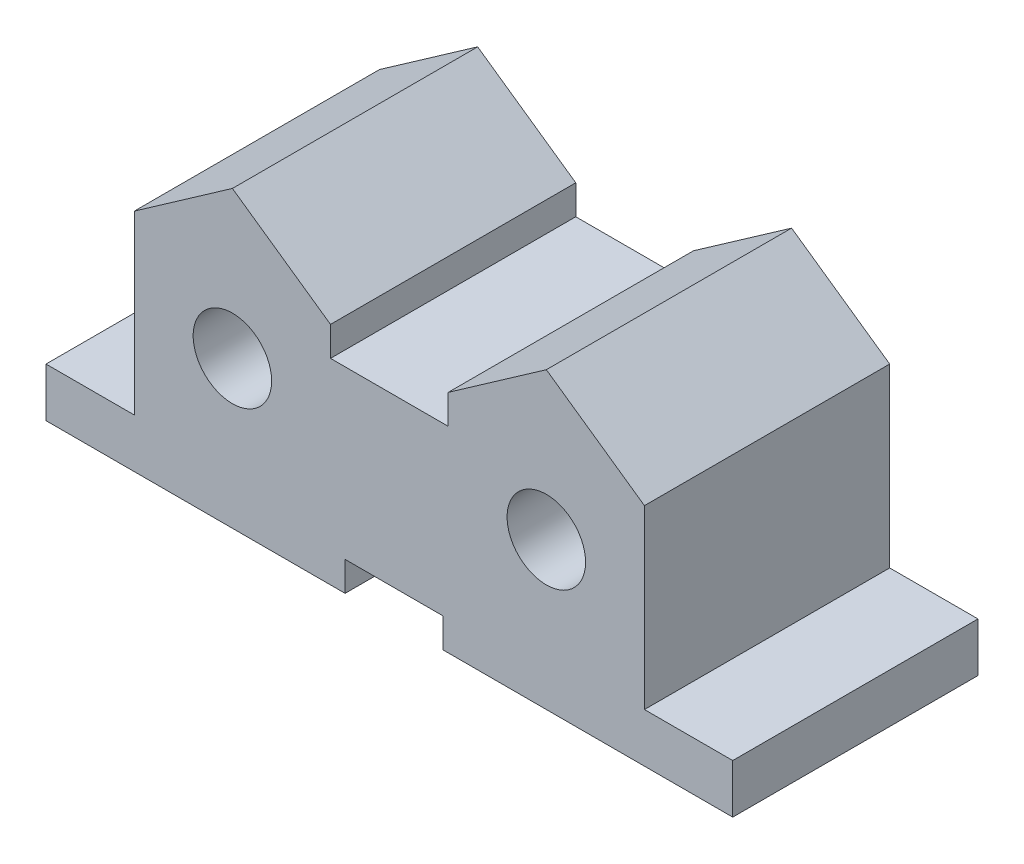
ISO-10303-21;
HEADER;
FILE_DESCRIPTION(('STEP AP214'),'2;1');
FILE_NAME('part.step','',(''),(''),'','','');
FILE_SCHEMA(('AUTOMOTIVE_DESIGN { 1 0 10303 214 1 1 1 1 }'));
ENDSEC;
DATA;
#1=APPLICATION_CONTEXT('core data for automotive mechanical design processes');
#2=APPLICATION_PROTOCOL_DEFINITION('international standard','automotive_design',2000,#1);
#3=PRODUCT_CONTEXT('',#1,'mechanical');
#4=PRODUCT('Part','Part','',(#3));
#5=PRODUCT_RELATED_PRODUCT_CATEGORY('part','',(#4));
#6=PRODUCT_DEFINITION_FORMATION('','',#4);
#7=PRODUCT_DEFINITION_CONTEXT('part definition',#1,'design');
#8=PRODUCT_DEFINITION('design','',#6,#7);
#9=PRODUCT_DEFINITION_SHAPE('','',#8);
#10=(LENGTH_UNIT() NAMED_UNIT(*) SI_UNIT(.MILLI.,.METRE.));
#11=(NAMED_UNIT(*) PLANE_ANGLE_UNIT() SI_UNIT($,.RADIAN.));
#12=(NAMED_UNIT(*) SI_UNIT($,.STERADIAN.) SOLID_ANGLE_UNIT());
#13=UNCERTAINTY_MEASURE_WITH_UNIT(LENGTH_MEASURE(1.E-05),#10,'distance_accuracy_value','');
#14=(GEOMETRIC_REPRESENTATION_CONTEXT(3) GLOBAL_UNCERTAINTY_ASSIGNED_CONTEXT((#13)) GLOBAL_UNIT_ASSIGNED_CONTEXT((#10,
#11,#12)) REPRESENTATION_CONTEXT('',''));
#15=CARTESIAN_POINT('',(0.,0.,0.));
#16=DIRECTION('',(0.,0.,1.));
#17=DIRECTION('',(1.,0.,0.));
#18=AXIS2_PLACEMENT_3D('',#15,#16,#17);
#19=CARTESIAN_POINT('',(0.,0.,0.));
#20=DIRECTION('',(0.,-1.,0.));
#21=DIRECTION('',(0.,0.,-1.));
#22=AXIS2_PLACEMENT_3D('',#19,#20,#21);
#23=PLANE('',#22);
#24=DIRECTION('',(0.,0.,-1.));
#25=VECTOR('',#24,1.);
#26=CARTESIAN_POINT('',(30.488696345371,0.,0.));
#27=LINE('',#26,#25);
#28=CARTESIAN_POINT('',(30.488696345371,0.,0.));
#29=VERTEX_POINT('',#28);
#30=CARTESIAN_POINT('',(30.488696345371,0.,-25.));
#31=VERTEX_POINT('',#30);
#32=EDGE_CURVE('E50',#29,#31,#27,.T.);
#33=ORIENTED_EDGE('',*,*,#32,.F.);
#34=DIRECTION('',(1.,0.,0.));
#35=VECTOR('',#34,1.);
#36=CARTESIAN_POINT('',(70.,0.,0.));
#37=LINE('',#36,#35);
#38=CARTESIAN_POINT('',(0.,0.,0.));
#39=VERTEX_POINT('',#38);
#40=EDGE_CURVE('E189',#39,#29,#37,.T.);
#41=ORIENTED_EDGE('',*,*,#40,.F.);
#42=DIRECTION('',(0.,0.,1.));
#43=VECTOR('',#42,1.);
#44=CARTESIAN_POINT('',(0.,0.,0.));
#45=LINE('',#44,#43);
#46=CARTESIAN_POINT('',(0.,0.,-25.));
#47=VERTEX_POINT('',#46);
#48=EDGE_CURVE('E200',#47,#39,#45,.T.);
#49=ORIENTED_EDGE('',*,*,#48,.F.);
#50=DIRECTION('',(-1.,0.,0.));
#51=VECTOR('',#50,1.);
#52=CARTESIAN_POINT('',(0.,0.,-25.));
#53=LINE('',#52,#51);
#54=EDGE_CURVE('E198',#31,#47,#53,.T.);
#55=ORIENTED_EDGE('',*,*,#54,.F.);
#56=EDGE_LOOP('',(#33,#41,#49,#55));
#57=FACE_BOUND('',#56,.T.);
#58=ADVANCED_FACE('F39',(#57),#23,.T.);
#59=CARTESIAN_POINT('',(0.,5.,0.));
#60=DIRECTION('',(0.,-1.,0.));
#61=DIRECTION('',(0.,0.,-1.));
#62=AXIS2_PLACEMENT_3D('',#59,#60,#61);
#63=PLANE('',#62);
#64=DIRECTION('',(0.,0.,1.));
#65=VECTOR('',#64,1.);
#66=CARTESIAN_POINT('',(9.,5.,-25.));
#67=LINE('',#66,#65);
#68=CARTESIAN_POINT('',(9.,5.,-25.));
#69=VERTEX_POINT('',#68);
#70=CARTESIAN_POINT('',(9.,5.,0.));
#71=VERTEX_POINT('',#70);
#72=EDGE_CURVE('E186',#69,#71,#67,.T.);
#73=ORIENTED_EDGE('',*,*,#72,.F.);
#74=DIRECTION('',(-1.,0.,0.));
#75=VECTOR('',#74,1.);
#76=CARTESIAN_POINT('',(0.,5.,-25.));
#77=LINE('',#76,#75);
#78=CARTESIAN_POINT('',(0.,5.,-25.));
#79=VERTEX_POINT('',#78);
#80=EDGE_CURVE('E249',#69,#79,#77,.T.);
#81=ORIENTED_EDGE('',*,*,#80,.T.);
#82=DIRECTION('',(0.,0.,1.));
#83=VECTOR('',#82,1.);
#84=CARTESIAN_POINT('',(0.,5.,0.));
#85=LINE('',#84,#83);
#86=CARTESIAN_POINT('',(0.,5.,0.));
#87=VERTEX_POINT('',#86);
#88=EDGE_CURVE('E193',#79,#87,#85,.T.);
#89=ORIENTED_EDGE('',*,*,#88,.T.);
#90=DIRECTION('',(1.,0.,0.));
#91=VECTOR('',#90,1.);
#92=CARTESIAN_POINT('',(70.,5.,0.));
#93=LINE('',#92,#91);
#94=EDGE_CURVE('E244',#87,#71,#93,.T.);
#95=ORIENTED_EDGE('',*,*,#94,.T.);
#96=EDGE_LOOP('',(#73,#81,#89,#95));
#97=FACE_BOUND('',#96,.T.);
#98=ADVANCED_FACE('F259',(#97),#63,.F.);
#99=CARTESIAN_POINT('',(70.,5.,0.));
#100=DIRECTION('',(0.,0.,-1.));
#101=DIRECTION('',(-1.,0.,0.));
#102=AXIS2_PLACEMENT_3D('',#99,#100,#101);
#103=PLANE('',#102);
#104=CARTESIAN_POINT('',(51.,15.,0.));
#105=DIRECTION('',(0.,0.,1.));
#106=DIRECTION('',(1.,0.,0.));
#107=AXIS2_PLACEMENT_3D('',#104,#105,#106);
#108=CIRCLE('',#107,4.00000000000001);
#109=CARTESIAN_POINT('',(55.,15.,0.));
#110=VERTEX_POINT('',#109);
#111=EDGE_CURVE('E216',#110,#110,#108,.T.);
#112=ORIENTED_EDGE('',*,*,#111,.F.);
#113=EDGE_LOOP('',(#112));
#114=FACE_BOUND('',#113,.T.);
#115=CARTESIAN_POINT('',(19.,15.,0.));
#116=DIRECTION('',(0.,0.,1.));
#117=DIRECTION('',(1.,0.,0.));
#118=AXIS2_PLACEMENT_3D('',#115,#116,#117);
#119=CIRCLE('',#118,4.);
#120=CARTESIAN_POINT('',(23.,15.,0.));
#121=VERTEX_POINT('',#120);
#122=EDGE_CURVE('E232',#121,#121,#119,.T.);
#123=ORIENTED_EDGE('',*,*,#122,.F.);
#124=EDGE_LOOP('',(#123));
#125=FACE_BOUND('',#124,.T.);
#126=ORIENTED_EDGE('',*,*,#40,.T.);
#127=DIRECTION('',(0.,-1.,0.));
#128=VECTOR('',#127,1.);
#129=CARTESIAN_POINT('',(30.488696345371,0.,0.));
#130=LINE('',#129,#128);
#131=CARTESIAN_POINT('',(30.488696345371,3.,0.));
#132=VERTEX_POINT('',#131);
#133=EDGE_CURVE('E221',#132,#29,#130,.T.);
#134=ORIENTED_EDGE('',*,*,#133,.F.);
#135=DIRECTION('',(-1.,0.,0.));
#136=VECTOR('',#135,1.);
#137=CARTESIAN_POINT('',(30.488696345371,3.,0.));
#138=LINE('',#137,#136);
#139=CARTESIAN_POINT('',(40.488696345371,3.,0.));
#140=VERTEX_POINT('',#139);
#141=EDGE_CURVE('E182',#140,#132,#138,.T.);
#142=ORIENTED_EDGE('',*,*,#141,.F.);
#143=DIRECTION('',(0.,1.,0.));
#144=VECTOR('',#143,1.);
#145=CARTESIAN_POINT('',(40.488696345371,3.,0.));
#146=LINE('',#145,#144);
#147=CARTESIAN_POINT('',(40.488696345371,0.,0.));
#148=VERTEX_POINT('',#147);
#149=EDGE_CURVE('E167',#148,#140,#146,.T.);
#150=ORIENTED_EDGE('',*,*,#149,.F.);
#151=CARTESIAN_POINT('',(70.,0.,0.));
#152=VERTEX_POINT('',#151);
#153=EDGE_CURVE('E180',#148,#152,#37,.T.);
#154=ORIENTED_EDGE('',*,*,#153,.T.);
#155=DIRECTION('',(0.,-1.,0.));
#156=VECTOR('',#155,1.);
#157=CARTESIAN_POINT('',(70.,5.,0.));
#158=LINE('',#157,#156);
#159=CARTESIAN_POINT('',(70.,5.,0.));
#160=VERTEX_POINT('',#159);
#161=EDGE_CURVE('E171',#160,#152,#158,.T.);
#162=ORIENTED_EDGE('',*,*,#161,.F.);
#163=CARTESIAN_POINT('',(61.,5.,0.));
#164=VERTEX_POINT('',#163);
#165=EDGE_CURVE('E203',#164,#160,#93,.T.);
#166=ORIENTED_EDGE('',*,*,#165,.F.);
#167=DIRECTION('',(0.,1.,0.));
#168=VECTOR('',#167,1.);
#169=CARTESIAN_POINT('',(61.,23.,0.));
#170=LINE('',#169,#168);
#171=CARTESIAN_POINT('',(61.,23.,0.));
#172=VERTEX_POINT('',#171);
#173=EDGE_CURVE('E61',#164,#172,#170,.T.);
#174=ORIENTED_EDGE('',*,*,#173,.T.);
#175=DIRECTION('',(-0.81923192051904,0.573462344363328,0.));
#176=VECTOR('',#175,1.);
#177=CARTESIAN_POINT('',(51.,30.,0.));
#178=LINE('',#177,#176);
#179=CARTESIAN_POINT('',(51.,30.,0.));
#180=VERTEX_POINT('',#179);
#181=EDGE_CURVE('E274',#172,#180,#178,.T.);
#182=ORIENTED_EDGE('',*,*,#181,.T.);
#183=DIRECTION('',(-0.81923192051904,-0.573462344363329,0.));
#184=VECTOR('',#183,1.);
#185=CARTESIAN_POINT('',(41.,23.,0.));
#186=LINE('',#185,#184);
#187=CARTESIAN_POINT('',(41.,23.,0.));
#188=VERTEX_POINT('',#187);
#189=EDGE_CURVE('E279',#180,#188,#186,.T.);
#190=ORIENTED_EDGE('',*,*,#189,.T.);
#191=DIRECTION('',(0.,-1.,0.));
#192=VECTOR('',#191,1.);
#193=CARTESIAN_POINT('',(41.,20.,0.));
#194=LINE('',#193,#192);
#195=CARTESIAN_POINT('',(41.,20.,0.));
#196=VERTEX_POINT('',#195);
#197=EDGE_CURVE('E284',#188,#196,#194,.T.);
#198=ORIENTED_EDGE('',*,*,#197,.T.);
#199=DIRECTION('',(-1.,0.,0.));
#200=VECTOR('',#199,1.);
#201=CARTESIAN_POINT('',(29.,20.,0.));
#202=LINE('',#201,#200);
#203=CARTESIAN_POINT('',(29.,20.,0.));
#204=VERTEX_POINT('',#203);
#205=EDGE_CURVE('E283',#196,#204,#202,.T.);
#206=ORIENTED_EDGE('',*,*,#205,.T.);
#207=DIRECTION('',(0.,1.,0.));
#208=VECTOR('',#207,1.);
#209=CARTESIAN_POINT('',(29.,23.,0.));
#210=LINE('',#209,#208);
#211=CARTESIAN_POINT('',(29.,23.,0.));
#212=VERTEX_POINT('',#211);
#213=EDGE_CURVE('E290',#204,#212,#210,.T.);
#214=ORIENTED_EDGE('',*,*,#213,.T.);
#215=DIRECTION('',(-0.81923192051904,0.573462344363328,0.));
#216=VECTOR('',#215,1.);
#217=CARTESIAN_POINT('',(19.,30.,0.));
#218=LINE('',#217,#216);
#219=CARTESIAN_POINT('',(19.,30.,0.));
#220=VERTEX_POINT('',#219);
#221=EDGE_CURVE('E286',#212,#220,#218,.T.);
#222=ORIENTED_EDGE('',*,*,#221,.T.);
#223=DIRECTION('',(-0.819231920519041,-0.573462344363328,0.));
#224=VECTOR('',#223,1.);
#225=CARTESIAN_POINT('',(9.,23.,0.));
#226=LINE('',#225,#224);
#227=CARTESIAN_POINT('',(9.,23.,0.));
#228=VERTEX_POINT('',#227);
#229=EDGE_CURVE('E291',#220,#228,#226,.T.);
#230=ORIENTED_EDGE('',*,*,#229,.T.);
#231=DIRECTION('',(0.,-1.,0.));
#232=VECTOR('',#231,1.);
#233=CARTESIAN_POINT('',(9.,5.,0.));
#234=LINE('',#233,#232);
#235=EDGE_CURVE('E243',#228,#71,#234,.T.);
#236=ORIENTED_EDGE('',*,*,#235,.T.);
#237=ORIENTED_EDGE('',*,*,#94,.F.);
#238=DIRECTION('',(0.,-1.,0.));
#239=VECTOR('',#238,1.);
#240=CARTESIAN_POINT('',(0.,5.,0.));
#241=LINE('',#240,#239);
#242=EDGE_CURVE('E205',#87,#39,#241,.T.);
#243=ORIENTED_EDGE('',*,*,#242,.T.);
#244=EDGE_LOOP('',(#126,#134,#142,#150,#154,#162,#166,#174,#182,#190,#198,#206,#214,#222,#230,
#236,#237,#243));
#245=FACE_BOUND('',#244,.T.);
#246=ADVANCED_FACE('F41',(#114,#125,#245),#103,.F.);
#247=CARTESIAN_POINT('',(70.,5.,-25.));
#248=DIRECTION('',(-1.,0.,0.));
#249=DIRECTION('',(0.,0.,1.));
#250=AXIS2_PLACEMENT_3D('',#247,#248,#249);
#251=PLANE('',#250);
#252=DIRECTION('',(0.,0.,-1.));
#253=VECTOR('',#252,1.);
#254=CARTESIAN_POINT('',(70.,0.,-25.));
#255=LINE('',#254,#253);
#256=CARTESIAN_POINT('',(70.,0.,-25.));
#257=VERTEX_POINT('',#256);
#258=EDGE_CURVE('E184',#152,#257,#255,.T.);
#259=ORIENTED_EDGE('',*,*,#258,.T.);
#260=DIRECTION('',(0.,-1.,0.));
#261=VECTOR('',#260,1.);
#262=CARTESIAN_POINT('',(70.,5.,-25.));
#263=LINE('',#262,#261);
#264=CARTESIAN_POINT('',(70.,5.,-25.));
#265=VERTEX_POINT('',#264);
#266=EDGE_CURVE('E208',#265,#257,#263,.T.);
#267=ORIENTED_EDGE('',*,*,#266,.F.);
#268=DIRECTION('',(0.,0.,-1.));
#269=VECTOR('',#268,1.);
#270=CARTESIAN_POINT('',(70.,5.,-25.));
#271=LINE('',#270,#269);
#272=EDGE_CURVE('E250',#160,#265,#271,.T.);
#273=ORIENTED_EDGE('',*,*,#272,.F.);
#274=ORIENTED_EDGE('',*,*,#161,.T.);
#275=EDGE_LOOP('',(#259,#267,#273,#274));
#276=FACE_BOUND('',#275,.T.);
#277=ADVANCED_FACE('F323',(#276),#251,.F.);
#278=CARTESIAN_POINT('',(0.,5.,-25.));
#279=DIRECTION('',(0.,0.,1.));
#280=DIRECTION('',(1.,0.,0.));
#281=AXIS2_PLACEMENT_3D('',#278,#279,#280);
#282=PLANE('',#281);
#283=CARTESIAN_POINT('',(51.,15.,-25.));
#284=DIRECTION('',(0.,0.,1.));
#285=DIRECTION('',(1.,0.,0.));
#286=AXIS2_PLACEMENT_3D('',#283,#284,#285);
#287=CIRCLE('',#286,4.00000000000001);
#288=CARTESIAN_POINT('',(55.,15.,-25.));
#289=VERTEX_POINT('',#288);
#290=EDGE_CURVE('E214',#289,#289,#287,.T.);
#291=ORIENTED_EDGE('',*,*,#290,.T.);
#292=EDGE_LOOP('',(#291));
#293=FACE_BOUND('',#292,.T.);
#294=CARTESIAN_POINT('',(19.,15.,-25.));
#295=DIRECTION('',(0.,0.,1.));
#296=DIRECTION('',(1.,0.,0.));
#297=AXIS2_PLACEMENT_3D('',#294,#295,#296);
#298=CIRCLE('',#297,4.);
#299=CARTESIAN_POINT('',(23.,15.,-25.));
#300=VERTEX_POINT('',#299);
#301=EDGE_CURVE('E215',#300,#300,#298,.T.);
#302=ORIENTED_EDGE('',*,*,#301,.T.);
#303=EDGE_LOOP('',(#302));
#304=FACE_BOUND('',#303,.T.);
#305=DIRECTION('',(-1.,0.,0.));
#306=VECTOR('',#305,1.);
#307=CARTESIAN_POINT('',(0.,3.,-25.));
#308=LINE('',#307,#306);
#309=CARTESIAN_POINT('',(40.488696345371,3.,-25.));
#310=VERTEX_POINT('',#309);
#311=CARTESIAN_POINT('',(30.488696345371,3.,-25.));
#312=VERTEX_POINT('',#311);
#313=EDGE_CURVE('E11',#310,#312,#308,.T.);
#314=ORIENTED_EDGE('',*,*,#313,.T.);
#315=DIRECTION('',(0.,-1.,0.));
#316=VECTOR('',#315,1.);
#317=CARTESIAN_POINT('',(30.488696345371,5.,-25.));
#318=LINE('',#317,#316);
#319=EDGE_CURVE('E225',#312,#31,#318,.T.);
#320=ORIENTED_EDGE('',*,*,#319,.T.);
#321=ORIENTED_EDGE('',*,*,#54,.T.);
#322=DIRECTION('',(0.,-1.,0.));
#323=VECTOR('',#322,1.);
#324=CARTESIAN_POINT('',(0.,5.,-25.));
#325=LINE('',#324,#323);
#326=EDGE_CURVE('E202',#79,#47,#325,.T.);
#327=ORIENTED_EDGE('',*,*,#326,.F.);
#328=ORIENTED_EDGE('',*,*,#80,.F.);
#329=DIRECTION('',(0.,-1.,0.));
#330=VECTOR('',#329,1.);
#331=CARTESIAN_POINT('',(9.,5.,-25.));
#332=LINE('',#331,#330);
#333=CARTESIAN_POINT('',(9.,23.,-25.));
#334=VERTEX_POINT('',#333);
#335=EDGE_CURVE('E265',#334,#69,#332,.T.);
#336=ORIENTED_EDGE('',*,*,#335,.F.);
#337=DIRECTION('',(-0.819231920519041,-0.573462344363328,0.));
#338=VECTOR('',#337,1.);
#339=CARTESIAN_POINT('',(9.,23.,-25.));
#340=LINE('',#339,#338);
#341=CARTESIAN_POINT('',(19.,30.,-25.));
#342=VERTEX_POINT('',#341);
#343=EDGE_CURVE('E264',#342,#334,#340,.T.);
#344=ORIENTED_EDGE('',*,*,#343,.F.);
#345=DIRECTION('',(-0.81923192051904,0.573462344363328,0.));
#346=VECTOR('',#345,1.);
#347=CARTESIAN_POINT('',(19.,30.,-25.));
#348=LINE('',#347,#346);
#349=CARTESIAN_POINT('',(29.,23.,-25.));
#350=VERTEX_POINT('',#349);
#351=EDGE_CURVE('E269',#350,#342,#348,.T.);
#352=ORIENTED_EDGE('',*,*,#351,.F.);
#353=DIRECTION('',(0.,1.,0.));
#354=VECTOR('',#353,1.);
#355=CARTESIAN_POINT('',(29.,23.,-25.));
#356=LINE('',#355,#354);
#357=CARTESIAN_POINT('',(29.,20.,-25.));
#358=VERTEX_POINT('',#357);
#359=EDGE_CURVE('E337',#358,#350,#356,.T.);
#360=ORIENTED_EDGE('',*,*,#359,.F.);
#361=DIRECTION('',(-1.,0.,0.));
#362=VECTOR('',#361,1.);
#363=CARTESIAN_POINT('',(29.,20.,-25.));
#364=LINE('',#363,#362);
#365=CARTESIAN_POINT('',(41.,20.,-25.));
#366=VERTEX_POINT('',#365);
#367=EDGE_CURVE('E336',#366,#358,#364,.T.);
#368=ORIENTED_EDGE('',*,*,#367,.F.);
#369=DIRECTION('',(0.,-1.,0.));
#370=VECTOR('',#369,1.);
#371=CARTESIAN_POINT('',(41.,20.,-25.));
#372=LINE('',#371,#370);
#373=CARTESIAN_POINT('',(41.,23.,-25.));
#374=VERTEX_POINT('',#373);
#375=EDGE_CURVE('E331',#374,#366,#372,.T.);
#376=ORIENTED_EDGE('',*,*,#375,.F.);
#377=DIRECTION('',(-0.81923192051904,-0.573462344363329,0.));
#378=VECTOR('',#377,1.);
#379=CARTESIAN_POINT('',(41.,23.,-25.));
#380=LINE('',#379,#378);
#381=CARTESIAN_POINT('',(51.,30.,-25.));
#382=VERTEX_POINT('',#381);
#383=EDGE_CURVE('E330',#382,#374,#380,.T.);
#384=ORIENTED_EDGE('',*,*,#383,.F.);
#385=DIRECTION('',(-0.81923192051904,0.573462344363328,0.));
#386=VECTOR('',#385,1.);
#387=CARTESIAN_POINT('',(51.,30.,-25.));
#388=LINE('',#387,#386);
#389=CARTESIAN_POINT('',(61.,23.,-25.));
#390=VERTEX_POINT('',#389);
#391=EDGE_CURVE('E324',#390,#382,#388,.T.);
#392=ORIENTED_EDGE('',*,*,#391,.F.);
#393=DIRECTION('',(0.,1.,0.));
#394=VECTOR('',#393,1.);
#395=CARTESIAN_POINT('',(61.,23.,-25.));
#396=LINE('',#395,#394);
#397=CARTESIAN_POINT('',(61.,5.,-25.));
#398=VERTEX_POINT('',#397);
#399=EDGE_CURVE('E293',#398,#390,#396,.T.);
#400=ORIENTED_EDGE('',*,*,#399,.F.);
#401=EDGE_CURVE('E255',#265,#398,#77,.T.);
#402=ORIENTED_EDGE('',*,*,#401,.F.);
#403=ORIENTED_EDGE('',*,*,#266,.T.);
#404=CARTESIAN_POINT('',(40.488696345371,0.,-25.));
#405=VERTEX_POINT('',#404);
#406=EDGE_CURVE('E197',#257,#405,#53,.T.);
#407=ORIENTED_EDGE('',*,*,#406,.T.);
#408=DIRECTION('',(0.,1.,0.));
#409=VECTOR('',#408,1.);
#410=CARTESIAN_POINT('',(40.488696345371,5.,-25.));
#411=LINE('',#410,#409);
#412=EDGE_CURVE('E53',#405,#310,#411,.T.);
#413=ORIENTED_EDGE('',*,*,#412,.T.);
#414=EDGE_LOOP('',(#314,#320,#321,#327,#328,#336,#344,#352,#360,#368,#376,#384,#392,#400,#402,
#403,#407,#413));
#415=FACE_BOUND('',#414,.T.);
#416=ADVANCED_FACE('F228',(#293,#304,#415),#282,.F.);
#417=CARTESIAN_POINT('',(0.,5.,0.));
#418=DIRECTION('',(1.,0.,0.));
#419=DIRECTION('',(0.,0.,-1.));
#420=AXIS2_PLACEMENT_3D('',#417,#418,#419);
#421=PLANE('',#420);
#422=ORIENTED_EDGE('',*,*,#48,.T.);
#423=ORIENTED_EDGE('',*,*,#242,.F.);
#424=ORIENTED_EDGE('',*,*,#88,.F.);
#425=ORIENTED_EDGE('',*,*,#326,.T.);
#426=EDGE_LOOP('',(#422,#423,#424,#425));
#427=FACE_BOUND('',#426,.T.);
#428=ADVANCED_FACE('F237',(#427),#421,.F.);
#429=ORIENTED_EDGE('',*,*,#401,.T.);
#430=DIRECTION('',(0.,0.,1.));
#431=VECTOR('',#430,1.);
#432=CARTESIAN_POINT('',(61.,5.,-25.));
#433=LINE('',#432,#431);
#434=EDGE_CURVE('E252',#398,#164,#433,.T.);
#435=ORIENTED_EDGE('',*,*,#434,.T.);
#436=ORIENTED_EDGE('',*,*,#165,.T.);
#437=ORIENTED_EDGE('',*,*,#272,.T.);
#438=EDGE_LOOP('',(#429,#435,#436,#437));
#439=FACE_BOUND('',#438,.T.);
#440=ADVANCED_FACE('F319',(#439),#63,.F.);
#441=DIRECTION('',(0.,0.,1.));
#442=VECTOR('',#441,1.);
#443=CARTESIAN_POINT('',(40.488696345371,0.,0.));
#444=LINE('',#443,#442);
#445=EDGE_CURVE('E162',#405,#148,#444,.T.);
#446=ORIENTED_EDGE('',*,*,#445,.F.);
#447=ORIENTED_EDGE('',*,*,#406,.F.);
#448=ORIENTED_EDGE('',*,*,#258,.F.);
#449=ORIENTED_EDGE('',*,*,#153,.F.);
#450=EDGE_LOOP('',(#446,#447,#448,#449));
#451=FACE_BOUND('',#450,.T.);
#452=ADVANCED_FACE('F181',(#451),#23,.T.);
#453=CARTESIAN_POINT('',(9.,5.,-25.));
#454=DIRECTION('',(-1.,0.,0.));
#455=DIRECTION('',(0.,0.,1.));
#456=AXIS2_PLACEMENT_3D('',#453,#454,#455);
#457=PLANE('',#456);
#458=ORIENTED_EDGE('',*,*,#235,.F.);
#459=DIRECTION('',(0.,0.,1.));
#460=VECTOR('',#459,1.);
#461=CARTESIAN_POINT('',(9.,23.,-25.));
#462=LINE('',#461,#460);
#463=EDGE_CURVE('E188',#334,#228,#462,.T.);
#464=ORIENTED_EDGE('',*,*,#463,.F.);
#465=ORIENTED_EDGE('',*,*,#335,.T.);
#466=ORIENTED_EDGE('',*,*,#72,.T.);
#467=EDGE_LOOP('',(#458,#464,#465,#466));
#468=FACE_BOUND('',#467,.T.);
#469=ADVANCED_FACE('F363',(#468),#457,.T.);
#470=CARTESIAN_POINT('',(9.,23.,-25.));
#471=DIRECTION('',(-0.573462344363328,0.819231920519041,0.));
#472=DIRECTION('',(-0.819231920519041,-0.573462344363328,0.));
#473=AXIS2_PLACEMENT_3D('',#470,#471,#472);
#474=PLANE('',#473);
#475=ORIENTED_EDGE('',*,*,#229,.F.);
#476=DIRECTION('',(0.,0.,1.));
#477=VECTOR('',#476,1.);
#478=CARTESIAN_POINT('',(19.,30.,-25.));
#479=LINE('',#478,#477);
#480=EDGE_CURVE('E300',#342,#220,#479,.T.);
#481=ORIENTED_EDGE('',*,*,#480,.F.);
#482=ORIENTED_EDGE('',*,*,#343,.T.);
#483=ORIENTED_EDGE('',*,*,#463,.T.);
#484=EDGE_LOOP('',(#475,#481,#482,#483));
#485=FACE_BOUND('',#484,.T.);
#486=ADVANCED_FACE('F362',(#485),#474,.T.);
#487=CARTESIAN_POINT('',(19.,30.,-25.));
#488=DIRECTION('',(0.573462344363328,0.81923192051904,0.));
#489=DIRECTION('',(-0.819231920519041,0.573462344363328,0.));
#490=AXIS2_PLACEMENT_3D('',#487,#488,#489);
#491=PLANE('',#490);
#492=ORIENTED_EDGE('',*,*,#221,.F.);
#493=DIRECTION('',(0.,0.,1.));
#494=VECTOR('',#493,1.);
#495=CARTESIAN_POINT('',(29.,23.,-25.));
#496=LINE('',#495,#494);
#497=EDGE_CURVE('E297',#350,#212,#496,.T.);
#498=ORIENTED_EDGE('',*,*,#497,.F.);
#499=ORIENTED_EDGE('',*,*,#351,.T.);
#500=ORIENTED_EDGE('',*,*,#480,.T.);
#501=EDGE_LOOP('',(#492,#498,#499,#500));
#502=FACE_BOUND('',#501,.T.);
#503=ADVANCED_FACE('F344',(#502),#491,.T.);
#504=CARTESIAN_POINT('',(29.,23.,-25.));
#505=DIRECTION('',(1.,0.,0.));
#506=DIRECTION('',(0.,0.,-1.));
#507=AXIS2_PLACEMENT_3D('',#504,#505,#506);
#508=PLANE('',#507);
#509=ORIENTED_EDGE('',*,*,#213,.F.);
#510=DIRECTION('',(0.,0.,1.));
#511=VECTOR('',#510,1.);
#512=CARTESIAN_POINT('',(29.,20.,-25.));
#513=LINE('',#512,#511);
#514=EDGE_CURVE('E305',#358,#204,#513,.T.);
#515=ORIENTED_EDGE('',*,*,#514,.F.);
#516=ORIENTED_EDGE('',*,*,#359,.T.);
#517=ORIENTED_EDGE('',*,*,#497,.T.);
#518=EDGE_LOOP('',(#509,#515,#516,#517));
#519=FACE_BOUND('',#518,.T.);
#520=ADVANCED_FACE('F348',(#519),#508,.T.);
#521=CARTESIAN_POINT('',(29.,20.,-25.));
#522=DIRECTION('',(0.,1.,0.));
#523=DIRECTION('',(0.,0.,1.));
#524=AXIS2_PLACEMENT_3D('',#521,#522,#523);
#525=PLANE('',#524);
#526=ORIENTED_EDGE('',*,*,#205,.F.);
#527=DIRECTION('',(0.,0.,1.));
#528=VECTOR('',#527,1.);
#529=CARTESIAN_POINT('',(41.,20.,-25.));
#530=LINE('',#529,#528);
#531=EDGE_CURVE('E304',#366,#196,#530,.T.);
#532=ORIENTED_EDGE('',*,*,#531,.F.);
#533=ORIENTED_EDGE('',*,*,#367,.T.);
#534=ORIENTED_EDGE('',*,*,#514,.T.);
#535=EDGE_LOOP('',(#526,#532,#533,#534));
#536=FACE_BOUND('',#535,.T.);
#537=ADVANCED_FACE('F355',(#536),#525,.T.);
#538=CARTESIAN_POINT('',(41.,20.,-25.));
#539=DIRECTION('',(-1.,0.,0.));
#540=DIRECTION('',(0.,-1.,0.));
#541=AXIS2_PLACEMENT_3D('',#538,#539,#540);
#542=PLANE('',#541);
#543=ORIENTED_EDGE('',*,*,#197,.F.);
#544=DIRECTION('',(0.,0.,1.));
#545=VECTOR('',#544,1.);
#546=CARTESIAN_POINT('',(41.,23.,-25.));
#547=LINE('',#546,#545);
#548=EDGE_CURVE('E308',#374,#188,#547,.T.);
#549=ORIENTED_EDGE('',*,*,#548,.F.);
#550=ORIENTED_EDGE('',*,*,#375,.T.);
#551=ORIENTED_EDGE('',*,*,#531,.T.);
#552=EDGE_LOOP('',(#543,#549,#550,#551));
#553=FACE_BOUND('',#552,.T.);
#554=ADVANCED_FACE('F360',(#553),#542,.T.);
#555=CARTESIAN_POINT('',(41.,23.,-25.));
#556=DIRECTION('',(-0.573462344363329,0.81923192051904,0.));
#557=DIRECTION('',(-0.81923192051904,-0.573462344363329,0.));
#558=AXIS2_PLACEMENT_3D('',#555,#556,#557);
#559=PLANE('',#558);
#560=ORIENTED_EDGE('',*,*,#189,.F.);
#561=DIRECTION('',(0.,0.,1.));
#562=VECTOR('',#561,1.);
#563=CARTESIAN_POINT('',(51.,30.,-25.));
#564=LINE('',#563,#562);
#565=EDGE_CURVE('E306',#382,#180,#564,.T.);
#566=ORIENTED_EDGE('',*,*,#565,.F.);
#567=ORIENTED_EDGE('',*,*,#383,.T.);
#568=ORIENTED_EDGE('',*,*,#548,.T.);
#569=EDGE_LOOP('',(#560,#566,#567,#568));
#570=FACE_BOUND('',#569,.T.);
#571=ADVANCED_FACE('F359',(#570),#559,.T.);
#572=CARTESIAN_POINT('',(51.,30.,-25.));
#573=DIRECTION('',(0.573462344363328,0.81923192051904,0.));
#574=DIRECTION('',(-0.81923192051904,0.573462344363328,0.));
#575=AXIS2_PLACEMENT_3D('',#572,#573,#574);
#576=PLANE('',#575);
#577=ORIENTED_EDGE('',*,*,#181,.F.);
#578=DIRECTION('',(0.,0.,1.));
#579=VECTOR('',#578,1.);
#580=CARTESIAN_POINT('',(61.,23.,-25.));
#581=LINE('',#580,#579);
#582=EDGE_CURVE('E267',#390,#172,#581,.T.);
#583=ORIENTED_EDGE('',*,*,#582,.F.);
#584=ORIENTED_EDGE('',*,*,#391,.T.);
#585=ORIENTED_EDGE('',*,*,#565,.T.);
#586=EDGE_LOOP('',(#577,#583,#584,#585));
#587=FACE_BOUND('',#586,.T.);
#588=ADVANCED_FACE('F316',(#587),#576,.T.);
#589=CARTESIAN_POINT('',(61.,23.,-25.));
#590=DIRECTION('',(1.,0.,0.));
#591=DIRECTION('',(0.,0.,-1.));
#592=AXIS2_PLACEMENT_3D('',#589,#590,#591);
#593=PLANE('',#592);
#594=ORIENTED_EDGE('',*,*,#173,.F.);
#595=ORIENTED_EDGE('',*,*,#434,.F.);
#596=ORIENTED_EDGE('',*,*,#399,.T.);
#597=ORIENTED_EDGE('',*,*,#582,.T.);
#598=EDGE_LOOP('',(#594,#595,#596,#597));
#599=FACE_BOUND('',#598,.T.);
#600=ADVANCED_FACE('F313',(#599),#593,.T.);
#601=CARTESIAN_POINT('',(19.,15.,-35.));
#602=DIRECTION('',(0.,0.,1.));
#603=DIRECTION('',(1.,0.,0.));
#604=AXIS2_PLACEMENT_3D('',#601,#602,#603);
#605=CYLINDRICAL_SURFACE('',#604,4.);
#606=ORIENTED_EDGE('',*,*,#122,.T.);
#607=EDGE_LOOP('',(#606));
#608=FACE_BOUND('',#607,.T.);
#609=ORIENTED_EDGE('',*,*,#301,.F.);
#610=EDGE_LOOP('',(#609));
#611=FACE_BOUND('',#610,.T.);
#612=ADVANCED_FACE('F391',(#608,#611),#605,.F.);
#613=CARTESIAN_POINT('',(51.,15.,-35.));
#614=DIRECTION('',(0.,0.,1.));
#615=DIRECTION('',(1.,0.,0.));
#616=AXIS2_PLACEMENT_3D('',#613,#614,#615);
#617=CYLINDRICAL_SURFACE('',#616,4.00000000000001);
#618=ORIENTED_EDGE('',*,*,#111,.T.);
#619=EDGE_LOOP('',(#618));
#620=FACE_BOUND('',#619,.T.);
#621=ORIENTED_EDGE('',*,*,#290,.F.);
#622=EDGE_LOOP('',(#621));
#623=FACE_BOUND('',#622,.T.);
#624=ADVANCED_FACE('F440',(#620,#623),#617,.F.);
#625=CARTESIAN_POINT('',(30.488696345371,3.,-35.));
#626=DIRECTION('',(0.,1.,0.));
#627=DIRECTION('',(0.,0.,1.));
#628=AXIS2_PLACEMENT_3D('',#625,#626,#627);
#629=PLANE('',#628);
#630=DIRECTION('',(0.,0.,1.));
#631=VECTOR('',#630,1.);
#632=CARTESIAN_POINT('',(40.488696345371,3.,-35.));
#633=LINE('',#632,#631);
#634=EDGE_CURVE('E477',#310,#140,#633,.T.);
#635=ORIENTED_EDGE('',*,*,#634,.T.);
#636=ORIENTED_EDGE('',*,*,#141,.T.);
#637=DIRECTION('',(0.,0.,1.));
#638=VECTOR('',#637,1.);
#639=CARTESIAN_POINT('',(30.488696345371,3.,-35.));
#640=LINE('',#639,#638);
#641=EDGE_CURVE('E481',#312,#132,#640,.T.);
#642=ORIENTED_EDGE('',*,*,#641,.F.);
#643=ORIENTED_EDGE('',*,*,#313,.F.);
#644=EDGE_LOOP('',(#635,#636,#642,#643));
#645=FACE_BOUND('',#644,.T.);
#646=ADVANCED_FACE('F443',(#645),#629,.F.);
#647=CARTESIAN_POINT('',(30.488696345371,0.,-35.));
#648=DIRECTION('',(-1.,0.,0.));
#649=DIRECTION('',(0.,0.,1.));
#650=AXIS2_PLACEMENT_3D('',#647,#648,#649);
#651=PLANE('',#650);
#652=ORIENTED_EDGE('',*,*,#641,.T.);
#653=ORIENTED_EDGE('',*,*,#133,.T.);
#654=ORIENTED_EDGE('',*,*,#32,.T.);
#655=ORIENTED_EDGE('',*,*,#319,.F.);
#656=EDGE_LOOP('',(#652,#653,#654,#655));
#657=FACE_BOUND('',#656,.T.);
#658=ADVANCED_FACE('F222',(#657),#651,.F.);
#659=CARTESIAN_POINT('',(40.488696345371,3.,-35.));
#660=DIRECTION('',(1.,0.,0.));
#661=DIRECTION('',(0.,0.,-1.));
#662=AXIS2_PLACEMENT_3D('',#659,#660,#661);
#663=PLANE('',#662);
#664=ORIENTED_EDGE('',*,*,#445,.T.);
#665=ORIENTED_EDGE('',*,*,#149,.T.);
#666=ORIENTED_EDGE('',*,*,#634,.F.);
#667=ORIENTED_EDGE('',*,*,#412,.F.);
#668=EDGE_LOOP('',(#664,#665,#666,#667));
#669=FACE_BOUND('',#668,.T.);
#670=ADVANCED_FACE('F164',(#669),#663,.F.);
#671=CLOSED_SHELL('',(#58,#98,#246,#277,#416,#428,#440,#452,#469,#486,#503,#520,#537,#554,#571,
#588,#600,#612,#624,#646,#658,#670));
#672=MANIFOLD_SOLID_BREP('B2',#671);
#673=ADVANCED_BREP_SHAPE_REPRESENTATION('',(#18,#672),#14);
#674=SHAPE_DEFINITION_REPRESENTATION(#9,#673);
ENDSEC;
END-ISO-10303-21;
